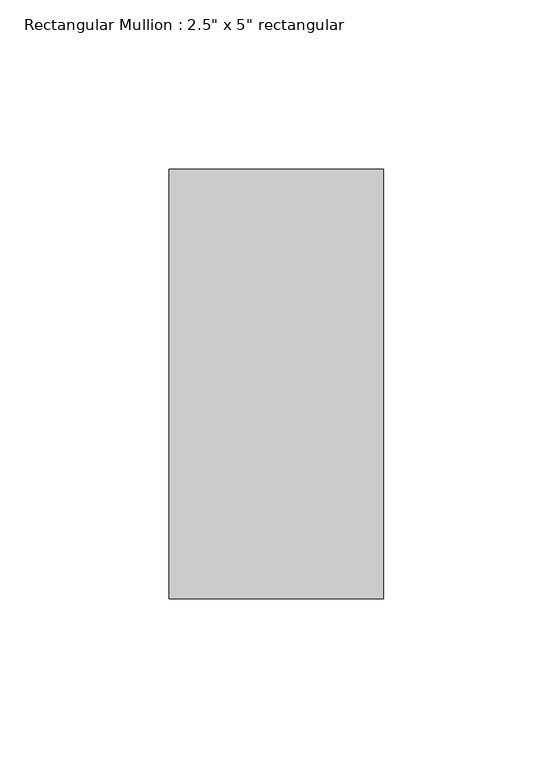
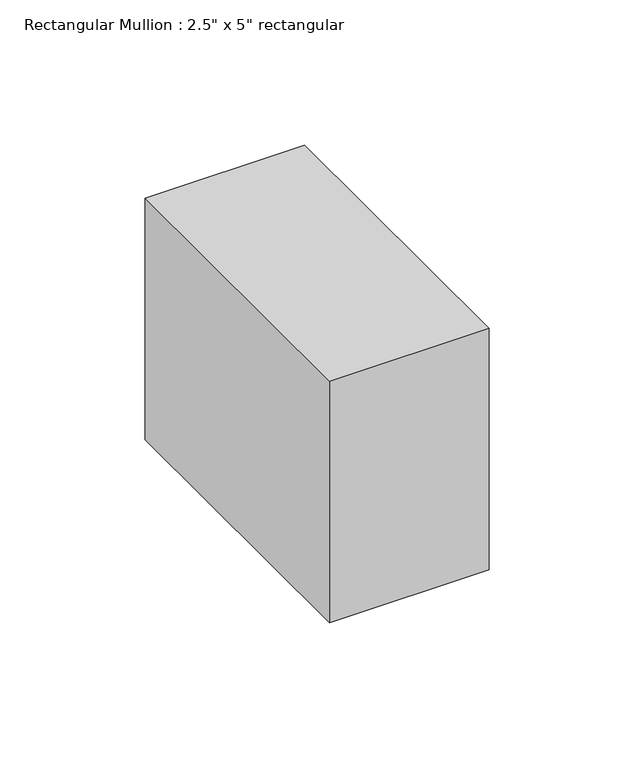
"""IFC4 building model written with IfcOpenShell, lengths in millimetres: member geometry."""

from ifc_helpers import new_model, si_unit, frame, origin, place, context, project, spatial, polyline, outline, extrude, source, transform, mapped, element, save


def member_cfc5edb3(model_context):
    return source(origin(), model_context, "Body", "SweptSolid", [
        extrude(outline(polyline([(31.75, 63.5), (31.75, -63.5), (-31.75, -63.5), (-31.75, 63.5), (31.75, 63.5)])), frame((0.0, 0.0, -101.6), z_axis=(0.0, 0.0, 1.0), x_axis=(1.0, 0.0, 0.0)), (0.0, 0.0, 1.0), 101.6),
    ])


if __name__ == "__main__":
    model = new_model("IFC4")
    model_context = context("Model", 3, world=origin())
    ifc_project = project(units=[si_unit("LENGTHUNIT", "METRE", prefix="MILLI")], contexts=[model_context])
    site = spatial("IfcSite", under=ifc_project)
    building = spatial("IfcBuilding", under=site)
    placement = place(None, origin())
    member_shape = member_cfc5edb3(model_context)
    element("IfcMember", 1, ObjectType="Rectangular Mullion : 2.5\" x 5\" rectangular", at=placement, inside=building, context=model_context, shape_type="MappedRepresentation", body=[
        mapped(member_shape, transform((0.0, 0.0, 0.0), x_axis=(1.0, 0.0, 0.0), y_axis=(0.0, 1.0, 0.0), z_axis=(0.0, 0.0, 1.0))),
    ])
    save(model, "model.ifc")

# Revit data of these elements
# Type "Rectangular Mullion : 2.5\" x 5\" rectangular"
#   built-in parameter 1007304 = 0.416667 (stored number, unit not read)
#   built-in parameter 1007301 = 0.104167 (stored number, unit not read)
#   built-in parameter 1007300 = 0.104167 (stored number, unit not read)
# Element 1 (IfcMember, "Rectangular Mullion : 2.5\" x 5\" rectangular")
#   Materials on its faces: "Aluminum"
# Materials
#   "Aluminum": class "Metal", colour RGB 247 247 247, transparency 0, Description = "Aluminum 6061", Cost = 0
